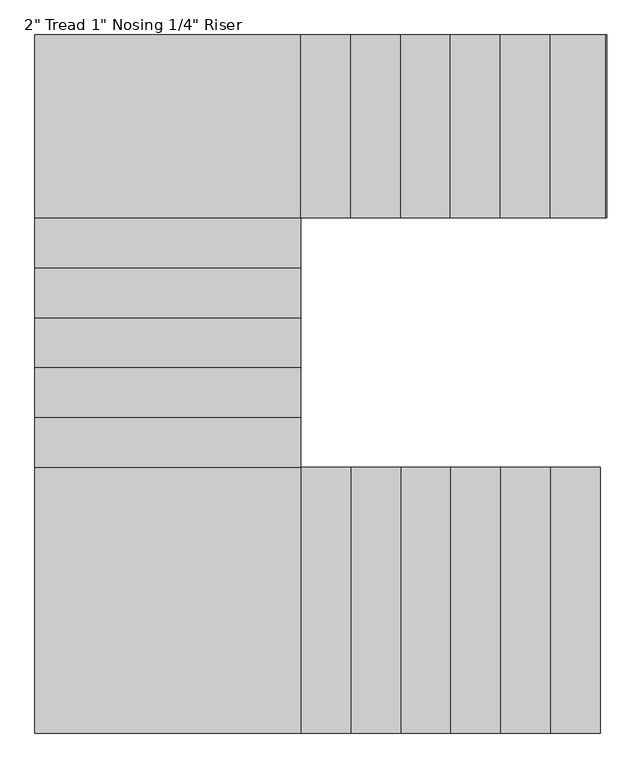
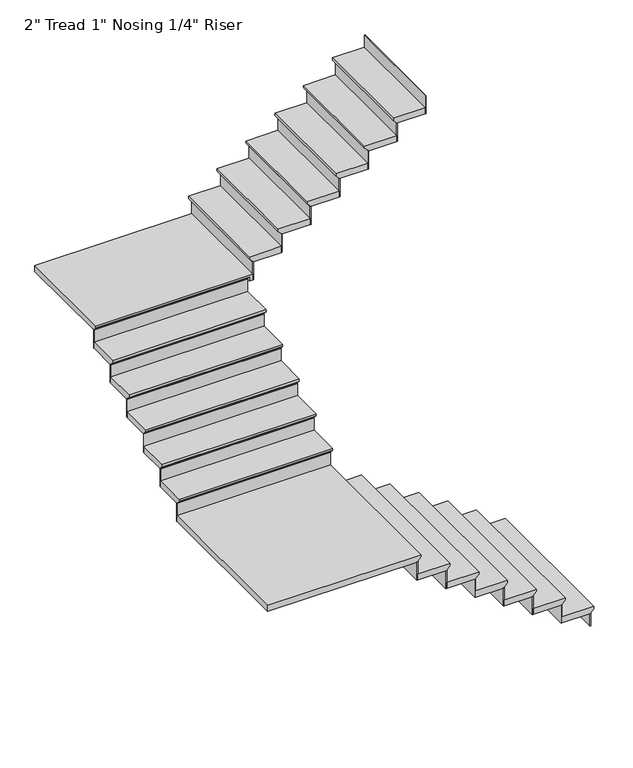
"""IFC4 building model written with IfcOpenShell, lengths in millimetres: stair flight geometry."""

from ifc_helpers import new_model, si_unit, origin, place, context, project, spatial, faceted_brep, source, transform, mapped, element, save


def stair_flight_217cdb56(model_context):
    return source(origin(), model_context, "Body", "Brep", [
        faceted_brep([(-2515.2117403, -5163.0426559, 6381.75), (-2515.2117403, -5163.0426559, 6400.8), (-2515.2117403, -6382.2426559, 6400.8), (-2515.2117403, -6382.2426559, 6381.75), (-2540.6117403, -5163.0426559, 6356.35), (-2540.6117403, -6382.2426559, 6356.35), (-2769.2117403, -5163.0426559, 6400.8), (-2769.2117403, -6382.2426559, 6400.8), (-2540.6117403, -6382.2426559, 6350.0), (-2769.2117403, -6382.2426559, 6350.0), (-2769.2117403, -5163.0426559, 6350.0), (-2540.6117403, -5163.0426559, 6350.0)], [[[0, 1, 2, 3]], [[4, 0, 3, 5]], [[2, 1, 6, 7]], [[8, 9, 10, 11]], [[2, 7, 9, 8, 5, 3]], [[8, 11, 4, 5]], [[6, 1, 0, 4, 11, 10]], [[7, 6, 10, 9]]]),
        faceted_brep([(-2540.6117403, -5163.0426559, 6350.0), (-2540.6117403, -5163.0426559, 6248.4), (-2546.9617403, -5163.0426559, 6248.4), (-2546.9617403, -5163.0426559, 6350.0), (-2540.6117403, -6382.2426559, 6350.0), (-2546.9617403, -6382.2426559, 6350.0), (-2546.9617403, -6382.2426559, 6248.4), (-2540.6117403, -6382.2426559, 6248.4)], [[[0, 1, 2, 3]], [[4, 5, 6, 7]], [[1, 0, 4, 7]], [[2, 1, 7, 6]], [[3, 2, 6, 5]], [[0, 3, 5, 4]]]),
        faceted_brep([(-2769.2117403, -5163.0426559, 6502.4), (-2769.2117403, -5163.0426559, 6350.0), (-2775.5617403, -5163.0426559, 6350.0), (-2775.5617403, -5163.0426559, 6502.4), (-2769.2117403, -6382.2426559, 6502.4), (-2775.5617403, -6382.2426559, 6502.4), (-2775.5617403, -6382.2426559, 6350.0), (-2769.2117403, -6382.2426559, 6350.0)], [[[0, 1, 2, 3]], [[4, 5, 6, 7]], [[1, 0, 4, 7]], [[2, 1, 7, 6]], [[3, 2, 6, 5]], [[0, 3, 5, 4]]]),
        faceted_brep([(-2743.8117403, -6382.2426559, 6553.2), (-2743.8117403, -5163.0426559, 6553.2), (-2997.8117403, -5163.0426559, 6553.2), (-2997.8117403, -6382.2426559, 6553.2), (-2769.2117403, -6382.2426559, 6502.4), (-2997.8117403, -6382.2426559, 6502.4), (-2997.8117403, -5163.0426559, 6502.4), (-2769.2117403, -5163.0426559, 6502.4), (-2769.2117403, -6382.2426559, 6508.75), (-2743.8117403, -6382.2426559, 6534.15), (-2769.2117403, -5163.0426559, 6508.75), (-2743.8117403, -5163.0426559, 6534.15)], [[[0, 1, 2, 3]], [[4, 5, 6, 7]], [[0, 3, 5, 4, 8, 9]], [[4, 7, 10, 8]], [[2, 1, 11, 10, 7, 6]], [[3, 2, 6, 5]], [[11, 1, 0, 9]], [[10, 11, 9, 8]]]),
        faceted_brep([(-2997.8117403, -5163.0426559, 6654.8), (-2997.8117403, -5163.0426559, 6502.4), (-3004.1617403, -5163.0426559, 6502.4), (-3004.1617403, -5163.0426559, 6654.8), (-2997.8117403, -6382.2426559, 6654.8), (-3004.1617403, -6382.2426559, 6654.8), (-3004.1617403, -6382.2426559, 6502.4), (-2997.8117403, -6382.2426559, 6502.4)], [[[0, 1, 2, 3]], [[4, 5, 6, 7]], [[1, 0, 4, 7]], [[2, 1, 7, 6]], [[3, 2, 6, 5]], [[0, 3, 5, 4]]]),
        faceted_brep([(-2972.4117403, -6382.2426559, 6705.6), (-2972.4117403, -5163.0426559, 6705.6), (-3226.4117403, -5163.0426559, 6705.6), (-3226.4117403, -6382.2426559, 6705.6), (-2997.8117403, -6382.2426559, 6654.8), (-3226.4117403, -6382.2426559, 6654.8), (-3226.4117403, -5163.0426559, 6654.8), (-2997.8117403, -5163.0426559, 6654.8), (-2997.8117403, -6382.2426559, 6661.15), (-2972.4117403, -6382.2426559, 6686.55), (-2997.8117403, -5163.0426559, 6661.15), (-2972.4117403, -5163.0426559, 6686.55)], [[[0, 1, 2, 3]], [[4, 5, 6, 7]], [[0, 3, 5, 4, 8, 9]], [[4, 7, 10, 8]], [[2, 1, 11, 10, 7, 6]], [[3, 2, 6, 5]], [[11, 1, 0, 9]], [[10, 11, 9, 8]]]),
        faceted_brep([(-3226.4117403, -5163.0426559, 6807.2), (-3226.4117403, -5163.0426559, 6654.8), (-3232.7617403, -5163.0426559, 6654.8), (-3232.7617403, -5163.0426559, 6807.2), (-3226.4117403, -6382.2426559, 6807.2), (-3232.7617403, -6382.2426559, 6807.2), (-3232.7617403, -6382.2426559, 6654.8), (-3226.4117403, -6382.2426559, 6654.8)], [[[0, 1, 2, 3]], [[4, 5, 6, 7]], [[1, 0, 4, 7]], [[2, 1, 7, 6]], [[3, 2, 6, 5]], [[0, 3, 5, 4]]]),
        faceted_brep([(-3201.0117403, -6382.2426559, 6858.0), (-3201.0117403, -5163.0426559, 6858.0), (-3455.0117403, -5163.0426559, 6858.0), (-3455.0117403, -6382.2426559, 6858.0), (-3226.4117403, -6382.2426559, 6807.2), (-3455.0117403, -6382.2426559, 6807.2), (-3455.0117403, -5163.0426559, 6807.2), (-3226.4117403, -5163.0426559, 6807.2), (-3226.4117403, -6382.2426559, 6813.55), (-3201.0117403, -6382.2426559, 6838.95), (-3226.4117403, -5163.0426559, 6813.55), (-3201.0117403, -5163.0426559, 6838.95)], [[[0, 1, 2, 3]], [[4, 5, 6, 7]], [[0, 3, 5, 4, 8, 9]], [[4, 7, 10, 8]], [[2, 1, 11, 10, 7, 6]], [[3, 2, 6, 5]], [[11, 1, 0, 9]], [[10, 11, 9, 8]]]),
        faceted_brep([(-3455.0117403, -5163.0426559, 6959.6), (-3455.0117403, -5163.0426559, 6807.2), (-3461.3617403, -5163.0426559, 6807.2), (-3461.3617403, -5163.0426559, 6959.6), (-3455.0117403, -6382.2426559, 6959.6), (-3461.3617403, -6382.2426559, 6959.6), (-3461.3617403, -6382.2426559, 6807.2), (-3455.0117403, -6382.2426559, 6807.2)], [[[0, 1, 2, 3]], [[4, 5, 6, 7]], [[1, 0, 4, 7]], [[2, 1, 7, 6]], [[3, 2, 6, 5]], [[0, 3, 5, 4]]]),
        faceted_brep([(-3429.6117403, -6382.2426559, 7010.4), (-3429.6117403, -5163.0426559, 7010.4), (-3683.6117403, -5163.0426559, 7010.4), (-3683.6117403, -6382.2426559, 7010.4), (-3455.0117403, -6382.2426559, 6959.6), (-3683.6117403, -6382.2426559, 6959.6), (-3683.6117403, -5163.0426559, 6959.6), (-3455.0117403, -5163.0426559, 6959.6), (-3455.0117403, -6382.2426559, 6965.95), (-3429.6117403, -6382.2426559, 6991.35), (-3455.0117403, -5163.0426559, 6965.95), (-3429.6117403, -5163.0426559, 6991.35)], [[[0, 1, 2, 3]], [[4, 5, 6, 7]], [[0, 3, 5, 4, 8, 9]], [[4, 7, 10, 8]], [[2, 1, 11, 10, 7, 6]], [[3, 2, 6, 5]], [[11, 1, 0, 9]], [[10, 11, 9, 8]]]),
        faceted_brep([(-3683.6117403, -5163.0426559, 7112.0), (-3683.6117403, -5163.0426559, 6959.6), (-3689.9617403, -5163.0426559, 6959.6), (-3689.9617403, -5163.0426559, 7112.0), (-3683.6117403, -6382.2426559, 7112.0), (-3689.9617403, -6382.2426559, 7112.0), (-3689.9617403, -6382.2426559, 6959.6), (-3683.6117403, -6382.2426559, 6959.6)], [[[0, 1, 2, 3]], [[4, 5, 6, 7]], [[1, 0, 4, 7]], [[2, 1, 7, 6]], [[3, 2, 6, 5]], [[0, 3, 5, 4]]]),
        faceted_brep([(-3658.2117403, -6382.2426559, 7162.8), (-3658.2117403, -5163.0426559, 7162.8), (-3912.2117403, -5163.0426559, 7162.8), (-3912.2117403, -6382.2426559, 7162.8), (-3683.6117403, -6382.2426559, 7112.0), (-3912.2117403, -6382.2426559, 7112.0), (-3912.2117403, -5163.0426559, 7112.0), (-3683.6117403, -5163.0426559, 7112.0), (-3683.6117403, -6382.2426559, 7118.35), (-3658.2117403, -6382.2426559, 7143.75), (-3683.6117403, -5163.0426559, 7118.35), (-3658.2117403, -5163.0426559, 7143.75)], [[[0, 1, 2, 3]], [[4, 5, 6, 7]], [[0, 3, 5, 4, 8, 9]], [[4, 7, 10, 8]], [[2, 1, 11, 10, 7, 6]], [[3, 2, 6, 5]], [[11, 1, 0, 9]], [[10, 11, 9, 8]]]),
        faceted_brep([(-3912.2117403, -5163.0426559, 7264.4), (-3912.2117403, -5163.0426559, 7112.0), (-3918.5617403, -5163.0426559, 7112.0), (-3918.5617403, -5163.0426559, 7264.4), (-3912.2117403, -6382.2426559, 7264.4), (-3918.5617403, -6382.2426559, 7264.4), (-3918.5617403, -6382.2426559, 7112.0), (-3912.2117403, -6382.2426559, 7112.0)], [[[0, 1, 2, 3]], [[4, 5, 6, 7]], [[1, 0, 4, 7]], [[2, 1, 7, 6]], [[3, 2, 6, 5]], [[0, 3, 5, 4]]]),
        faceted_brep([(-5106.0117403, -5137.6426559, 7315.2), (-5106.0117403, -6382.2426559, 7315.2), (-3886.8117403, -6382.2426559, 7315.2), (-3886.8117403, -5137.6426559, 7315.2), (-5106.0117403, -6382.2426559, 7264.4), (-5106.0117403, -5137.6426559, 7264.4), (-3886.8117403, -5137.6426559, 7264.4), (-3886.8117403, -5163.0426559, 7264.4), (-3912.2117403, -5163.0426559, 7264.4), (-3912.2117403, -6382.2426559, 7264.4), (-3912.2117403, -6382.2426559, 7270.75), (-3886.8117403, -6382.2426559, 7296.15), (-3912.2117403, -5163.0426559, 7270.75), (-3886.8117403, -5163.0426559, 7296.15)], [[[0, 1, 2, 3]], [[4, 5, 6, 7, 8, 9]], [[1, 0, 5, 4]], [[2, 1, 4, 9, 10, 11]], [[9, 8, 12, 10]], [[8, 7, 13, 12]], [[3, 2, 11, 13, 7, 6]], [[0, 3, 6, 5]], [[11, 10, 12, 13]]]),
        faceted_brep([(-3886.8117403, -5137.6426559, 7416.8), (-3886.8117403, -5137.6426559, 7264.4), (-3886.8117403, -5131.2926559, 7264.4), (-3886.8117403, -5131.2926559, 7416.8), (-5106.0117403, -5137.6426559, 7416.8), (-5106.0117403, -5131.2926559, 7416.8), (-5106.0117403, -5131.2926559, 7264.4), (-5106.0117403, -5137.6426559, 7264.4)], [[[0, 1, 2, 3]], [[4, 5, 6, 7]], [[1, 0, 4, 7]], [[2, 1, 7, 6]], [[3, 2, 6, 5]], [[0, 3, 5, 4]]]),
        faceted_brep([(-5106.0117403, -5163.0426559, 7467.6), (-3886.8117403, -5163.0426559, 7467.6), (-3886.8117403, -4909.0426559, 7467.6), (-5106.0117403, -4909.0426559, 7467.6), (-5106.0117403, -5137.6426559, 7416.8), (-5106.0117403, -4909.0426559, 7416.8), (-3886.8117403, -4909.0426559, 7416.8), (-3886.8117403, -5137.6426559, 7416.8), (-5106.0117403, -5137.6426559, 7423.15), (-5106.0117403, -5163.0426559, 7448.55), (-3886.8117403, -5137.6426559, 7423.15), (-3886.8117403, -5163.0426559, 7448.55)], [[[0, 1, 2, 3]], [[4, 5, 6, 7]], [[0, 3, 5, 4, 8, 9]], [[4, 7, 10, 8]], [[2, 1, 11, 10, 7, 6]], [[3, 2, 6, 5]], [[11, 1, 0, 9]], [[10, 11, 9, 8]]]),
        faceted_brep([(-3886.8117403, -4909.0426559, 7569.2), (-3886.8117403, -4909.0426559, 7416.8), (-3886.8117403, -4902.6926559, 7416.8), (-3886.8117403, -4902.6926559, 7569.2), (-5106.0117403, -4909.0426559, 7569.2), (-5106.0117403, -4902.6926559, 7569.2), (-5106.0117403, -4902.6926559, 7416.8), (-5106.0117403, -4909.0426559, 7416.8)], [[[0, 1, 2, 3]], [[4, 5, 6, 7]], [[1, 0, 4, 7]], [[2, 1, 7, 6]], [[3, 2, 6, 5]], [[0, 3, 5, 4]]]),
        faceted_brep([(-5106.0117403, -4934.4426559, 7620.0), (-3886.8117403, -4934.4426559, 7620.0), (-3886.8117403, -4680.4426559, 7620.0), (-5106.0117403, -4680.4426559, 7620.0), (-5106.0117403, -4909.0426559, 7569.2), (-5106.0117403, -4680.4426559, 7569.2), (-3886.8117403, -4680.4426559, 7569.2), (-3886.8117403, -4909.0426559, 7569.2), (-5106.0117403, -4909.0426559, 7575.55), (-5106.0117403, -4934.4426559, 7600.95), (-3886.8117403, -4909.0426559, 7575.55), (-3886.8117403, -4934.4426559, 7600.95)], [[[0, 1, 2, 3]], [[4, 5, 6, 7]], [[0, 3, 5, 4, 8, 9]], [[4, 7, 10, 8]], [[2, 1, 11, 10, 7, 6]], [[3, 2, 6, 5]], [[11, 1, 0, 9]], [[10, 11, 9, 8]]]),
        faceted_brep([(-3886.8117403, -4680.4426559, 7721.6), (-3886.8117403, -4680.4426559, 7569.2), (-3886.8117403, -4674.0926559, 7569.2), (-3886.8117403, -4674.0926559, 7721.6), (-5106.0117403, -4680.4426559, 7721.6), (-5106.0117403, -4674.0926559, 7721.6), (-5106.0117403, -4674.0926559, 7569.2), (-5106.0117403, -4680.4426559, 7569.2)], [[[0, 1, 2, 3]], [[4, 5, 6, 7]], [[1, 0, 4, 7]], [[2, 1, 7, 6]], [[3, 2, 6, 5]], [[0, 3, 5, 4]]]),
        faceted_brep([(-5106.0117403, -4705.8426559, 7772.4), (-3886.8117403, -4705.8426559, 7772.4), (-3886.8117403, -4451.8426559, 7772.4), (-5106.0117403, -4451.8426559, 7772.4), (-5106.0117403, -4680.4426559, 7721.6), (-5106.0117403, -4451.8426559, 7721.6), (-3886.8117403, -4451.8426559, 7721.6), (-3886.8117403, -4680.4426559, 7721.6), (-5106.0117403, -4680.4426559, 7727.95), (-5106.0117403, -4705.8426559, 7753.35), (-3886.8117403, -4680.4426559, 7727.95), (-3886.8117403, -4705.8426559, 7753.35)], [[[0, 1, 2, 3]], [[4, 5, 6, 7]], [[0, 3, 5, 4, 8, 9]], [[4, 7, 10, 8]], [[2, 1, 11, 10, 7, 6]], [[3, 2, 6, 5]], [[11, 1, 0, 9]], [[10, 11, 9, 8]]]),
        faceted_brep([(-3886.8117403, -4451.8426559, 7874.0), (-3886.8117403, -4451.8426559, 7721.6), (-3886.8117403, -4445.4926559, 7721.6), (-3886.8117403, -4445.4926559, 7874.0), (-5106.0117403, -4451.8426559, 7874.0), (-5106.0117403, -4445.4926559, 7874.0), (-5106.0117403, -4445.4926559, 7721.6), (-5106.0117403, -4451.8426559, 7721.6)], [[[0, 1, 2, 3]], [[4, 5, 6, 7]], [[1, 0, 4, 7]], [[2, 1, 7, 6]], [[3, 2, 6, 5]], [[0, 3, 5, 4]]]),
        faceted_brep([(-5106.0117403, -4477.2426559, 7924.8), (-3886.8117403, -4477.2426559, 7924.8), (-3886.8117403, -4223.2426559, 7924.8), (-5106.0117403, -4223.2426559, 7924.8), (-5106.0117403, -4451.8426559, 7874.0), (-5106.0117403, -4223.2426559, 7874.0), (-3886.8117403, -4223.2426559, 7874.0), (-3886.8117403, -4451.8426559, 7874.0), (-5106.0117403, -4451.8426559, 7880.35), (-5106.0117403, -4477.2426559, 7905.75), (-3886.8117403, -4451.8426559, 7880.35), (-3886.8117403, -4477.2426559, 7905.75)], [[[0, 1, 2, 3]], [[4, 5, 6, 7]], [[0, 3, 5, 4, 8, 9]], [[4, 7, 10, 8]], [[2, 1, 11, 10, 7, 6]], [[3, 2, 6, 5]], [[11, 1, 0, 9]], [[10, 11, 9, 8]]]),
        faceted_brep([(-3886.8117403, -4223.2426559, 8026.4), (-3886.8117403, -4223.2426559, 7874.0), (-3886.8117403, -4216.8926559, 7874.0), (-3886.8117403, -4216.8926559, 8026.4), (-5106.0117403, -4223.2426559, 8026.4), (-5106.0117403, -4216.8926559, 8026.4), (-5106.0117403, -4216.8926559, 7874.0), (-5106.0117403, -4223.2426559, 7874.0)], [[[0, 1, 2, 3]], [[4, 5, 6, 7]], [[1, 0, 4, 7]], [[2, 1, 7, 6]], [[3, 2, 6, 5]], [[0, 3, 5, 4]]]),
        faceted_brep([(-5106.0117403, -4248.6426559, 8077.2), (-3886.8117403, -4248.6426559, 8077.2), (-3886.8117403, -3994.6426559, 8077.2), (-5106.0117403, -3994.6426559, 8077.2), (-5106.0117403, -4223.2426559, 8026.4), (-5106.0117403, -3994.6426559, 8026.4), (-3886.8117403, -3994.6426559, 8026.4), (-3886.8117403, -4223.2426559, 8026.4), (-5106.0117403, -4223.2426559, 8032.75), (-5106.0117403, -4248.6426559, 8058.15), (-3886.8117403, -4223.2426559, 8032.75), (-3886.8117403, -4248.6426559, 8058.15)], [[[0, 1, 2, 3]], [[4, 5, 6, 7]], [[0, 3, 5, 4, 8, 9]], [[4, 7, 10, 8]], [[2, 1, 11, 10, 7, 6]], [[3, 2, 6, 5]], [[11, 1, 0, 9]], [[10, 11, 9, 8]]]),
        faceted_brep([(-3886.8117403, -3994.6426559, 8178.8), (-3886.8117403, -3994.6426559, 8026.4), (-3886.8117403, -3988.2926559, 8026.4), (-3886.8117403, -3988.2926559, 8178.8), (-5106.0117403, -3994.6426559, 8178.8), (-5106.0117403, -3988.2926559, 8178.8), (-5106.0117403, -3988.2926559, 8026.4), (-5106.0117403, -3994.6426559, 8026.4)], [[[0, 1, 2, 3]], [[4, 5, 6, 7]], [[1, 0, 4, 7]], [[2, 1, 7, 6]], [[3, 2, 6, 5]], [[0, 3, 5, 4]]]),
        faceted_brep([(-3861.4117403, -3181.8426559, 8229.6), (-5106.0117403, -3181.8426559, 8229.6), (-5106.0117403, -4020.0426559, 8229.6), (-3861.4117403, -4020.0426559, 8229.6), (-5106.0117403, -3181.8426559, 8178.8), (-3861.4117403, -3181.8426559, 8178.8), (-3861.4117403, -4020.0426559, 8178.8), (-3886.8117403, -4020.0426559, 8178.8), (-3886.8117403, -3994.6426559, 8178.8), (-5106.0117403, -3994.6426559, 8178.8), (-5106.0117403, -3994.6426559, 8185.15), (-5106.0117403, -4020.0426559, 8210.55), (-3886.8117403, -3994.6426559, 8185.15), (-3886.8117403, -4020.0426559, 8210.55)], [[[0, 1, 2, 3]], [[4, 5, 6, 7, 8, 9]], [[1, 0, 5, 4]], [[2, 1, 4, 9, 10, 11]], [[9, 8, 12, 10]], [[8, 7, 13, 12]], [[3, 2, 11, 13, 7, 6]], [[0, 3, 6, 5]], [[11, 10, 12, 13]]]),
        faceted_brep([(-3861.4117403, -4020.0426559, 8331.2), (-3861.4117403, -4020.0426559, 8178.8), (-3855.0617403, -4020.0426559, 8178.8), (-3855.0617403, -4020.0426559, 8331.2), (-3861.4117403, -3181.8426559, 8331.2), (-3855.0617403, -3181.8426559, 8331.2), (-3855.0617403, -3181.8426559, 8178.8), (-3861.4117403, -3181.8426559, 8178.8)], [[[0, 1, 2, 3]], [[4, 5, 6, 7]], [[1, 0, 4, 7]], [[2, 1, 7, 6]], [[3, 2, 6, 5]], [[0, 3, 5, 4]]]),
        faceted_brep([(-3886.8117403, -3181.8426559, 8382.0), (-3886.8117403, -4020.0426559, 8382.0), (-3632.8117403, -4020.0426559, 8382.0), (-3632.8117403, -3181.8426559, 8382.0), (-3861.4117403, -3181.8426559, 8331.2), (-3632.8117403, -3181.8426559, 8331.2), (-3632.8117403, -4020.0426559, 8331.2), (-3861.4117403, -4020.0426559, 8331.2), (-3861.4117403, -3181.8426559, 8337.55), (-3886.8117403, -3181.8426559, 8362.95), (-3861.4117403, -4020.0426559, 8337.55), (-3886.8117403, -4020.0426559, 8362.95)], [[[0, 1, 2, 3]], [[4, 5, 6, 7]], [[0, 3, 5, 4, 8, 9]], [[4, 7, 10, 8]], [[2, 1, 11, 10, 7, 6]], [[3, 2, 6, 5]], [[11, 1, 0, 9]], [[10, 11, 9, 8]]]),
        faceted_brep([(-3632.8117403, -4020.0426559, 8483.6), (-3632.8117403, -4020.0426559, 8331.2), (-3626.4617403, -4020.0426559, 8331.2), (-3626.4617403, -4020.0426559, 8483.6), (-3632.8117403, -3181.8426559, 8483.6), (-3626.4617403, -3181.8426559, 8483.6), (-3626.4617403, -3181.8426559, 8331.2), (-3632.8117403, -3181.8426559, 8331.2)], [[[0, 1, 2, 3]], [[4, 5, 6, 7]], [[1, 0, 4, 7]], [[2, 1, 7, 6]], [[3, 2, 6, 5]], [[0, 3, 5, 4]]]),
        faceted_brep([(-3658.2117403, -3181.8426559, 8534.4), (-3658.2117403, -4020.0426559, 8534.4), (-3404.2117403, -4020.0426559, 8534.4), (-3404.2117403, -3181.8426559, 8534.4), (-3632.8117403, -3181.8426559, 8483.6), (-3404.2117403, -3181.8426559, 8483.6), (-3404.2117403, -4020.0426559, 8483.6), (-3632.8117403, -4020.0426559, 8483.6), (-3632.8117403, -3181.8426559, 8489.95), (-3658.2117403, -3181.8426559, 8515.35), (-3632.8117403, -4020.0426559, 8489.95), (-3658.2117403, -4020.0426559, 8515.35)], [[[0, 1, 2, 3]], [[4, 5, 6, 7]], [[0, 3, 5, 4, 8, 9]], [[4, 7, 10, 8]], [[2, 1, 11, 10, 7, 6]], [[3, 2, 6, 5]], [[11, 1, 0, 9]], [[10, 11, 9, 8]]]),
        faceted_brep([(-3404.2117403, -4020.0426559, 8636.0), (-3404.2117403, -4020.0426559, 8483.6), (-3397.8617403, -4020.0426559, 8483.6), (-3397.8617403, -4020.0426559, 8636.0), (-3404.2117403, -3181.8426559, 8636.0), (-3397.8617403, -3181.8426559, 8636.0), (-3397.8617403, -3181.8426559, 8483.6), (-3404.2117403, -3181.8426559, 8483.6)], [[[0, 1, 2, 3]], [[4, 5, 6, 7]], [[1, 0, 4, 7]], [[2, 1, 7, 6]], [[3, 2, 6, 5]], [[0, 3, 5, 4]]]),
        faceted_brep([(-3429.6117403, -3181.8426559, 8686.8), (-3429.6117403, -4020.0426559, 8686.8), (-3175.6117403, -4020.0426559, 8686.8), (-3175.6117403, -3181.8426559, 8686.8), (-3404.2117403, -3181.8426559, 8636.0), (-3175.6117403, -3181.8426559, 8636.0), (-3175.6117403, -4020.0426559, 8636.0), (-3404.2117403, -4020.0426559, 8636.0), (-3404.2117403, -3181.8426559, 8642.35), (-3429.6117403, -3181.8426559, 8667.75), (-3404.2117403, -4020.0426559, 8642.35), (-3429.6117403, -4020.0426559, 8667.75)], [[[0, 1, 2, 3]], [[4, 5, 6, 7]], [[0, 3, 5, 4, 8, 9]], [[4, 7, 10, 8]], [[2, 1, 11, 10, 7, 6]], [[3, 2, 6, 5]], [[11, 1, 0, 9]], [[10, 11, 9, 8]]]),
        faceted_brep([(-3175.6117403, -4020.0426559, 8788.4), (-3175.6117403, -4020.0426559, 8636.0), (-3169.2617403, -4020.0426559, 8636.0), (-3169.2617403, -4020.0426559, 8788.4), (-3175.6117403, -3181.8426559, 8788.4), (-3169.2617403, -3181.8426559, 8788.4), (-3169.2617403, -3181.8426559, 8636.0), (-3175.6117403, -3181.8426559, 8636.0)], [[[0, 1, 2, 3]], [[4, 5, 6, 7]], [[1, 0, 4, 7]], [[2, 1, 7, 6]], [[3, 2, 6, 5]], [[0, 3, 5, 4]]]),
        faceted_brep([(-3201.0117403, -3181.8426559, 8839.2), (-3201.0117403, -4020.0426559, 8839.2), (-2947.0117403, -4020.0426559, 8839.2), (-2947.0117403, -3181.8426559, 8839.2), (-3175.6117403, -3181.8426559, 8788.4), (-2947.0117403, -3181.8426559, 8788.4), (-2947.0117403, -4020.0426559, 8788.4), (-3175.6117403, -4020.0426559, 8788.4), (-3175.6117403, -3181.8426559, 8794.75), (-3201.0117403, -3181.8426559, 8820.15), (-3175.6117403, -4020.0426559, 8794.75), (-3201.0117403, -4020.0426559, 8820.15)], [[[0, 1, 2, 3]], [[4, 5, 6, 7]], [[0, 3, 5, 4, 8, 9]], [[4, 7, 10, 8]], [[2, 1, 11, 10, 7, 6]], [[3, 2, 6, 5]], [[11, 1, 0, 9]], [[10, 11, 9, 8]]]),
        faceted_brep([(-2947.0117403, -4020.0426559, 8940.8), (-2947.0117403, -4020.0426559, 8788.4), (-2940.6617403, -4020.0426559, 8788.4), (-2940.6617403, -4020.0426559, 8940.8), (-2947.0117403, -3181.8426559, 8940.8), (-2940.6617403, -3181.8426559, 8940.8), (-2940.6617403, -3181.8426559, 8788.4), (-2947.0117403, -3181.8426559, 8788.4)], [[[0, 1, 2, 3]], [[4, 5, 6, 7]], [[1, 0, 4, 7]], [[2, 1, 7, 6]], [[3, 2, 6, 5]], [[0, 3, 5, 4]]]),
        faceted_brep([(-2972.4117403, -3181.8426559, 8991.6), (-2972.4117403, -4020.0426559, 8991.6), (-2718.4117403, -4020.0426559, 8991.6), (-2718.4117403, -3181.8426559, 8991.6), (-2947.0117403, -3181.8426559, 8940.8), (-2718.4117403, -3181.8426559, 8940.8), (-2718.4117403, -4020.0426559, 8940.8), (-2947.0117403, -4020.0426559, 8940.8), (-2947.0117403, -3181.8426559, 8947.15), (-2972.4117403, -3181.8426559, 8972.55), (-2947.0117403, -4020.0426559, 8947.15), (-2972.4117403, -4020.0426559, 8972.55)], [[[0, 1, 2, 3]], [[4, 5, 6, 7]], [[0, 3, 5, 4, 8, 9]], [[4, 7, 10, 8]], [[2, 1, 11, 10, 7, 6]], [[3, 2, 6, 5]], [[11, 1, 0, 9]], [[10, 11, 9, 8]]]),
        faceted_brep([(-2718.4117403, -4020.0426559, 9093.2), (-2718.4117403, -4020.0426559, 8940.8), (-2712.0617403, -4020.0426559, 8940.8), (-2712.0617403, -4020.0426559, 9093.2), (-2718.4117403, -3181.8426559, 9093.2), (-2712.0617403, -3181.8426559, 9093.2), (-2712.0617403, -3181.8426559, 8940.8), (-2718.4117403, -3181.8426559, 8940.8)], [[[0, 1, 2, 3]], [[4, 5, 6, 7]], [[1, 0, 4, 7]], [[2, 1, 7, 6]], [[3, 2, 6, 5]], [[0, 3, 5, 4]]]),
        faceted_brep([(-2489.8117403, -4020.0426559, 9245.6), (-2489.8117403, -4020.0426559, 9093.2), (-2483.4617403, -4020.0426559, 9093.2), (-2483.4617403, -4020.0426559, 9245.6), (-2489.8117403, -3181.8426559, 9245.6), (-2483.4617403, -3181.8426559, 9245.6), (-2483.4617403, -3181.8426559, 9093.2), (-2489.8117403, -3181.8426559, 9093.2)], [[[0, 1, 2, 3]], [[4, 5, 6, 7]], [[1, 0, 4, 7]], [[2, 1, 7, 6]], [[3, 2, 6, 5]], [[0, 3, 5, 4]]]),
        faceted_brep([(-2743.8117403, -3181.8426559, 9144.0), (-2743.8117403, -4020.0426559, 9144.0), (-2489.8117403, -4020.0426559, 9144.0), (-2489.8117403, -3181.8426559, 9144.0), (-2718.4117403, -3181.8426559, 9093.2), (-2489.8117403, -3181.8426559, 9093.2), (-2489.8117403, -4020.0426559, 9093.2), (-2718.4117403, -4020.0426559, 9093.2), (-2718.4117403, -3181.8426559, 9099.55), (-2743.8117403, -3181.8426559, 9124.95), (-2718.4117403, -4020.0426559, 9099.55), (-2743.8117403, -4020.0426559, 9124.95)], [[[0, 1, 2, 3]], [[4, 5, 6, 7]], [[0, 3, 5, 4, 8, 9]], [[4, 7, 10, 8]], [[2, 1, 11, 10, 7, 6]], [[3, 2, 6, 5]], [[11, 1, 0, 9]], [[10, 11, 9, 8]]]),
    ])


if __name__ == "__main__":
    model = new_model("IFC4")
    model_context = context("Model", 3, world=origin())
    ifc_project = project(units=[si_unit("LENGTHUNIT", "METRE", prefix="MILLI")], contexts=[model_context])
    site = spatial("IfcSite", under=ifc_project)
    building = spatial("IfcBuilding", under=site)
    placement = place(None, origin())
    stair_flight_shape = stair_flight_217cdb56(model_context)
    element("IfcStairFlight", 1, ObjectType="2\" Tread 1\" Nosing 1/4\" Riser", at=placement, inside=building, context=model_context, shape_type="MappedRepresentation", body=[
        mapped(stair_flight_shape, transform((0.0, 0.0, 0.0), x_axis=(1.0, 0.0, 0.0), y_axis=(0.0, 1.0, 0.0), z_axis=(0.0, 0.0, 1.0))),
    ])
    save(model, "model.ifc")

# Revit data of these elements
# Element 1 (IfcStairFlight, "2\" Tread 1\" Nosing 1/4\" Riser")
#   Materials on its faces: "Wood Planks"
# Materials
#   "Wood Planks": class "Wood", colour RGB 193 160 115, transparency 0, Description = "Physical material.", Cost = 0
